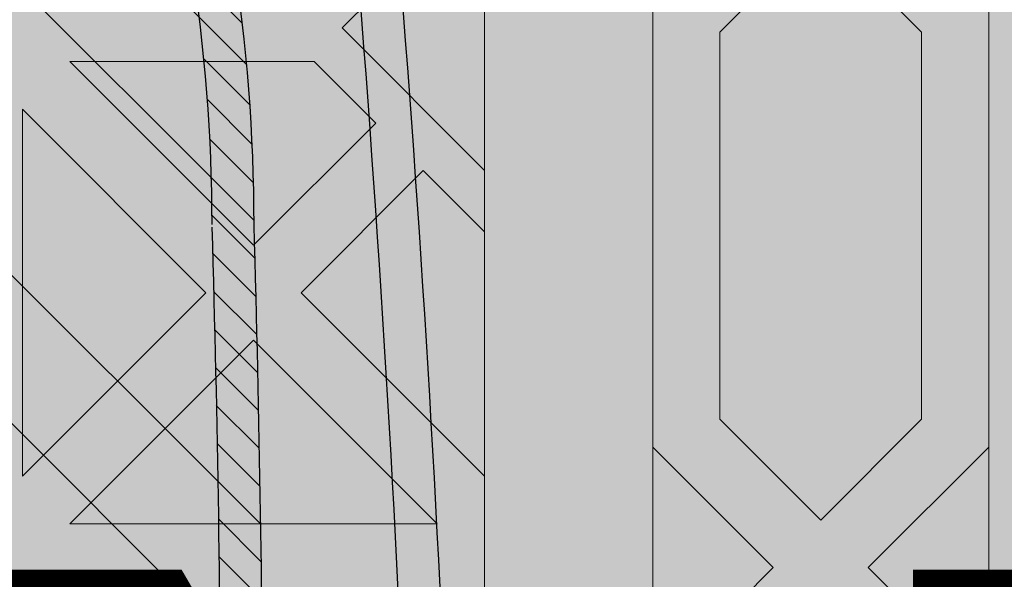
# Model space of a CAD drawing. Units: inches. Extents: x 844 to 2234, y 346 to 1084.
# Tile 84 of 93: x 2006.557 to 2010.294, y 704.373 to 706.497. Entities that reach past the tile are written whole.
import ezdxf

# ---------------------------------------------------------------- set-up
doc = ezdxf.new("R2010")
doc.units = ezdxf.units.IN
doc.header["$MEASUREMENT"] = 0
for name, color, linetype, lineweight in [('A-ANNO-DIMS', 2, 'Continuous', 18), ('furniture', 8, 'Continuous', 18), ('RA-AP-01$0$INT', 35, 'Continuous', 5)]:
    doc.layers.add(name, color=color, linetype=linetype, lineweight=lineweight)
doc.layers.add('RA-AP-01$0$FURN', color=3, linetype='Continuous')
doc.layers.add('RA-AP-01$0$WOOD', color=64, linetype='Continuous')
doc.styles.get("Standard").update_dxf_attribs({"font": 'arial.ttf'})
doc.dimstyles.get("Standard").update_dxf_attribs({"dimtxt": 6, "dimasz": 3, "dimexe": 0.18, "dimexo": 0.0625, "dimgap": 0.09, "dimtad": 0, "dimtih": 1, "dimtoh": 1, "dimdec": 1, "dimzin": 0, "dimdsep": 46, "dimlunit": 3, "dimtxsty": 'Standard', "dimblk": 'ARCHTICK', "dimcen": 0.09, "dimadec": 0, "dimazin": 0, "dimtfac": 1, "dimtdec": 1, "dimtofl": 0, "dimtmove": 0, "dimatfit": 3, "dimfxl": 1, "dimtolj": 1, "dimtzin": 0, "dimarcsym": 0})

# ---------------------------------------------------------------- blocks, each defined once
blk = doc.blocks.new('A$C18D01794')
at = {"layer": 'RA-AP-01$0$INT'}
h = blk.add_hatch(color=256, dxfattribs=at)
h.paths.add_polyline_path([(4.35521, -6.15671), (4.35521, -8.05671), (5.45521, -8.05671), (5.45521, -6.15671)])
h.paths.add_polyline_path([(4.40521, -8.00671), (4.40521, -6.20671), (5.40521, -6.20671), (5.40521, -8.00671)], flags=16)
h = blk.add_hatch(color=256, dxfattribs=at)
h.paths.add_polyline_path([(4.50521, -7.5855), (4.46935, -7.54964), (4.50521, -7.51378), (4.50521, -7.38196), (4.46935, -7.34611), (4.50521, -7.31025), (4.50521, -7.17843), (4.46935, -7.14257), (4.50521, -7.10671), (4.47692, -7.10671), (4.45521, -7.12843), (4.43349, -7.10671), (4.40521, -7.10671), (4.44106, -7.14257), (4.40521, -7.17843), (4.40521, -7.31025), (4.44106, -7.34611), (4.40521, -7.38196), (4.40521, -7.51378), (4.44106, -7.54964), (4.40521, -7.5855), (4.40521, -7.71732), (4.44106, -7.75318), (4.40521, -7.78903), (4.40521, -8.00671), (4.64435, -8.00671), (4.68021, -7.97085), (4.71606, -8.00671), (4.86935, -8.00671), (4.90521, -7.97085), (4.94106, -8.00671), (5.09435, -8.00671), (5.13021, -7.97085), (5.16606, -8.00671), (5.40521, -8.00671), (5.40521, -7.78903), (5.36935, -7.75318), (5.40521, -7.71732), (5.40521, -7.5855), (5.36935, -7.54964), (5.40521, -7.51378), (5.40521, -7.38196), (5.36935, -7.34611), (5.40521, -7.31025), (5.40521, -7.17843), (5.36935, -7.14257), (5.40521, -7.10671), (5.37692, -7.10671), (5.35521, -7.12843), (5.33349, -7.10671), (5.30521, -7.10671), (5.34106, -7.14257), (5.30521, -7.17843), (5.30521, -7.31025), (5.34106, -7.34611), (5.30521, -7.38196), (5.30521, -7.51378), (5.34106, -7.54964), (5.30521, -7.5855), (5.30521, -7.71732), (5.34106, -7.75318), (5.30521, -7.78903), (5.30521, -7.90671), (5.16606, -7.90671), (5.13021, -7.94257), (5.09435, -7.90671), (4.94106, -7.90671), (4.90521, -7.94257), (4.86935, -7.90671), (4.71606, -7.90671), (4.68021, -7.94257), (4.64435, -7.90671), (4.50521, -7.90671), (4.50521, -7.78903), (4.46935, -7.75318), (4.50521, -7.71732)])
h.paths.add_polyline_path([(4.48521, -7.70903), (4.45521, -7.73903), (4.42521, -7.70903), (4.42521, -7.59378), (4.45521, -7.56378), (4.48521, -7.59378)], flags=16)
h.paths.add_polyline_path([(4.45521, -7.76732), (4.48521, -7.79732), (4.48521, -7.91257), (4.45521, -7.94257), (4.42521, -7.91257), (4.42521, -7.79732)], flags=16)
h.paths.add_polyline_path([(4.45521, -7.5355), (4.42521, -7.5055), (4.42521, -7.39025), (4.45521, -7.36025), (4.48521, -7.39025), (4.48521, -7.5055)], flags=16)
h.paths.add_polyline_path([(4.49935, -7.92671), (4.63606, -7.92671), (4.66606, -7.95671), (4.63606, -7.98671), (4.49935, -7.98671), (4.46935, -7.95671)], flags=16)
h.paths.add_polyline_path([(4.42521, -7.94085), (4.47106, -7.98671), (4.42521, -7.98671)], flags=16)
h.paths.add_polyline_path([(4.45521, -7.33196), (4.42521, -7.30196), (4.42521, -7.18671), (4.45521, -7.15671), (4.48521, -7.18671), (4.48521, -7.30196)], flags=16)
h.paths.add_polyline_path([(4.72435, -7.92671), (4.86106, -7.92671), (4.89106, -7.95671), (4.86106, -7.98671), (4.72435, -7.98671), (4.69435, -7.95671)], flags=16)
h.paths.add_polyline_path([(4.91935, -7.95671), (4.94935, -7.92671), (5.08606, -7.92671), (5.11606, -7.95671), (5.08606, -7.98671), (4.94935, -7.98671)], flags=16)
h.paths.add_polyline_path([(5.14435, -7.95671), (5.17435, -7.92671), (5.31106, -7.92671), (5.34106, -7.95671), (5.31106, -7.98671), (5.17435, -7.98671)], flags=16)
h.paths.add_polyline_path([(5.32521, -7.59378), (5.35521, -7.56378), (5.38521, -7.59378), (5.38521, -7.70903), (5.35521, -7.73903), (5.32521, -7.70903)], flags=16)
h.paths.add_polyline_path([(5.32521, -7.79732), (5.35521, -7.76732), (5.38521, -7.79732), (5.38521, -7.91257), (5.35521, -7.94257), (5.32521, -7.91257)], flags=16)
h.paths.add_polyline_path([(5.32521, -7.5055), (5.32521, -7.39025), (5.35521, -7.36025), (5.38521, -7.39025), (5.38521, -7.5055), (5.35521, -7.5355)], flags=16)
h.paths.add_polyline_path([(5.32521, -7.30196), (5.32521, -7.18671), (5.35521, -7.15671), (5.38521, -7.18671), (5.38521, -7.30196), (5.35521, -7.33196)], flags=16)
h.paths.add_polyline_path([(5.33935, -7.98671), (5.38521, -7.94085), (5.38521, -7.98671)], flags=16)
h = blk.add_hatch(color=256, dxfattribs=at)
h.paths.add_polyline_path([(4.46935, -7.14257), (4.50521, -7.17843), (4.50521, -7.10671)])
h.paths.add_polyline_path([(4.45521, -7.12843), (4.47692, -7.10671), (4.43349, -7.10671)])
h.paths.add_polyline_path([(4.40521, -7.17843), (4.44106, -7.14257), (4.40521, -7.10671)])
h.paths.add_polyline_path([(4.42521, -7.30196), (4.45521, -7.33196), (4.48521, -7.30196), (4.48521, -7.18671), (4.45521, -7.15671), (4.42521, -7.18671)])
h.paths.add_polyline_path([(4.50521, -7.38196), (4.50521, -7.31025), (4.46935, -7.34611)])
h.paths.add_polyline_path([(4.42521, -7.5055), (4.45521, -7.5355), (4.48521, -7.5055), (4.48521, -7.39025), (4.45521, -7.36025), (4.42521, -7.39025)])
h.paths.add_polyline_path([(4.42521, -7.70903), (4.45521, -7.73903), (4.48521, -7.70903), (4.48521, -7.59378), (4.45521, -7.56378), (4.42521, -7.59378)])
h.paths.add_polyline_path([(4.46935, -7.54964), (4.50521, -7.5855), (4.50521, -7.51378)])
h.paths.add_polyline_path([(4.40521, -7.5855), (4.44106, -7.54964), (4.40521, -7.51378)])
h.paths.add_polyline_path([(4.40521, -7.78903), (4.44106, -7.75318), (4.40521, -7.71732)])
h.paths.add_polyline_path([(4.46935, -7.75318), (4.50521, -7.78903), (4.50521, -7.71732)])
h.paths.add_polyline_path([(4.42521, -7.91257), (4.45521, -7.94257), (4.48521, -7.91257), (4.48521, -7.79732), (4.45521, -7.76732), (4.42521, -7.79732)])
h.paths.add_polyline_path([(4.42521, -7.98671), (4.47106, -7.98671), (4.42521, -7.94085)])
h.paths.add_polyline_path([(4.49935, -7.98671), (4.63606, -7.98671), (4.66606, -7.95671), (4.63606, -7.92671), (4.49935, -7.92671), (4.46935, -7.95671)])
h.paths.add_polyline_path([(4.68021, -7.94257), (4.71606, -7.90671), (4.64435, -7.90671)])
h.paths.add_polyline_path([(4.64435, -8.00671), (4.71606, -8.00671), (4.68021, -7.97085)])
h.paths.add_polyline_path([(4.72435, -7.98671), (4.86106, -7.98671), (4.89106, -7.95671), (4.86106, -7.92671), (4.72435, -7.92671), (4.69435, -7.95671)])
h.paths.add_polyline_path([(4.90521, -7.94257), (4.94106, -7.90671), (4.86935, -7.90671)])
h.paths.add_polyline_path([(4.86935, -8.00671), (4.94106, -8.00671), (4.90521, -7.97085)])
h.paths.add_polyline_path([(4.94935, -7.98671), (5.08606, -7.98671), (5.11606, -7.95671), (5.08606, -7.92671), (4.94935, -7.92671), (4.91935, -7.95671)])
h.paths.add_polyline_path([(5.13021, -7.94257), (5.16606, -7.90671), (5.09435, -7.90671)])
h.paths.add_polyline_path([(5.09435, -8.00671), (5.16606, -8.00671), (5.13021, -7.97085)])
h.paths.add_polyline_path([(5.17435, -7.98671), (5.31106, -7.98671), (5.34106, -7.95671), (5.31106, -7.92671), (5.17435, -7.92671), (5.14435, -7.95671)])
h.paths.add_polyline_path([(5.32521, -7.91257), (5.35521, -7.94257), (5.38521, -7.91257), (5.38521, -7.79732), (5.35521, -7.76732), (5.32521, -7.79732)])
h.paths.add_polyline_path([(5.33935, -7.98671), (5.38521, -7.98671), (5.38521, -7.94085)])
h.paths.add_polyline_path([(5.32521, -7.70903), (5.35521, -7.73903), (5.38521, -7.70903), (5.38521, -7.59378), (5.35521, -7.56378), (5.32521, -7.59378)])
h.paths.add_polyline_path([(5.30521, -7.78903), (5.34106, -7.75318), (5.30521, -7.71732)])
h.paths.add_polyline_path([(5.36935, -7.75318), (5.40521, -7.78903), (5.40521, -7.71732)])
h.paths.add_polyline_path([(5.40521, -7.5855), (5.40521, -7.51378), (5.36935, -7.54964)])
h.paths.add_polyline_path([(5.30521, -7.5855), (5.34106, -7.54964), (5.30521, -7.51378)])
h.paths.add_polyline_path([(5.32521, -7.5055), (5.35521, -7.5355), (5.38521, -7.5055), (5.38521, -7.39025), (5.35521, -7.36025), (5.32521, -7.39025)])
h.paths.add_polyline_path([(5.30521, -7.38196), (5.34106, -7.34611), (5.30521, -7.31025)])
h.paths.add_polyline_path([(5.32521, -7.30196), (5.35521, -7.33196), (5.38521, -7.30196), (5.38521, -7.18671), (5.35521, -7.15671), (5.32521, -7.18671)])
h.paths.add_polyline_path([(5.40458, -7.38134, -0.001218), (5.40521, -7.38111), (5.40521, -7.31025), (5.36935, -7.34611)])
h.paths.add_polyline_path([(5.36935, -7.14257), (5.40521, -7.17843), (5.40521, -7.10671)])
h.paths.add_polyline_path([(5.35521, -7.12843), (5.37692, -7.10671), (5.33349, -7.10671)])
h.paths.add_polyline_path([(5.30521, -7.17843), (5.34106, -7.14257), (5.30521, -7.10671)])
for points in [[(4.50521, -7.90671), (5.30521, -7.90671), (5.30521, -7.10671), (5.25521, -7.10671), (5.25521, -7.85671), (4.55521, -7.85671), (4.55521, -7.10671), (4.50521, -7.10671)], [(4.40521, -7.38196), (4.44106, -7.34611), (4.40521, -7.31025)]]:
    blk.add_hatch(color=256, dxfattribs=at).paths.add_polyline_path(points)
h = blk.add_hatch(color=256, dxfattribs=at)
h.paths.add_polyline_path([(4.58592, -7.85671), (4.6142, -7.85671), (4.66885, -7.80207), (4.72349, -7.85671), (4.77177, -7.85671), (4.82642, -7.80207), (4.86278, -7.83843), (4.8445, -7.85671), (4.86278, -7.85671), (4.90521, -7.81429), (4.94763, -7.85671), (4.96592, -7.85671), (4.94763, -7.83843), (4.98399, -7.80207), (5.03864, -7.85671), (5.08692, -7.85671), (5.14157, -7.80207), (5.19621, -7.85671), (5.2245, -7.85671), (4.90521, -7.53742)])
h.paths.add_polyline_path([(4.89521, -7.57571), (4.89521, -7.685), (4.84056, -7.63035)], flags=16)
h.paths.add_polyline_path([(4.91521, -7.57571), (4.96985, -7.63035), (4.91521, -7.685)], flags=16)
h.paths.add_polyline_path([(4.82642, -7.64449), (4.88106, -7.69914), (4.77177, -7.69914)], flags=16)
h.paths.add_polyline_path([(4.98399, -7.64449), (5.03864, -7.69914), (4.92935, -7.69914)], flags=16)
h.paths.add_polyline_path([(4.88106, -7.71914), (4.82642, -7.77378), (4.77177, -7.71914)], flags=16)
h.paths.add_polyline_path([(4.92935, -7.71914), (5.03864, -7.71914), (4.98399, -7.77378)], flags=16)
h.paths.add_polyline_path([(4.89521, -7.73328), (4.89521, -7.806), (4.87692, -7.82429), (4.84056, -7.78793)], flags=16)
h.paths.add_polyline_path([(4.91521, -7.73328), (4.96985, -7.78793), (4.93349, -7.82429), (4.91521, -7.806)], flags=16)
h.paths.add_polyline_path([(4.75763, -7.73328), (4.81228, -7.78793), (4.75763, -7.84257)], flags=16)
h.paths.add_polyline_path([(4.73763, -7.73328), (4.73763, -7.84257), (4.68299, -7.78793)], flags=16)
h.paths.add_polyline_path([(5.05278, -7.73328), (5.05278, -7.84257), (4.99814, -7.78793)], flags=16)
h.paths.add_polyline_path([(5.07278, -7.73328), (5.12742, -7.78793), (5.07278, -7.84257)], flags=16)
h.paths.add_polyline_path([(4.93592, -7.50671), (5.25521, -7.826), (5.25521, -7.79772), (5.20056, -7.74307), (5.25521, -7.68843), (5.25521, -7.64014), (5.20056, -7.5855), (5.23692, -7.54914), (5.25521, -7.56742), (5.25521, -7.54914), (5.21278, -7.50671), (5.25521, -7.46429), (5.25521, -7.446), (5.23692, -7.46429), (5.20056, -7.42793), (5.25521, -7.37328), (5.25521, -7.325), (5.20056, -7.27035), (5.25521, -7.21571), (5.25521, -7.18742)])
h.paths.add_polyline_path([(5.04299, -7.42793), (5.09763, -7.37328), (5.09763, -7.48257)], flags=16)
h.paths.add_polyline_path([(5.02885, -7.44207), (5.08349, -7.49671), (4.9742, -7.49671)], flags=16)
h.paths.add_polyline_path([(5.11763, -7.37328), (5.17228, -7.42793), (5.11763, -7.48257)], flags=16)
h.paths.add_polyline_path([(5.08349, -7.51671), (5.02885, -7.57136), (4.9742, -7.51671)], flags=16)
h.paths.add_polyline_path([(5.13177, -7.35914), (5.18642, -7.41378), (5.24106, -7.35914)], flags=17)
h.paths.add_polyline_path([(5.13177, -7.49671), (5.18642, -7.44207), (5.22278, -7.47843), (5.2045, -7.49671)], flags=16)
h.paths.add_polyline_path([(5.09763, -7.53085), (5.09763, -7.64014), (5.04299, -7.5855)], flags=16)
h.paths.add_polyline_path([(5.13177, -7.33914), (5.24106, -7.33914), (5.18642, -7.28449)], flags=17)
h.paths.add_polyline_path([(5.13177, -7.51671), (5.2045, -7.51671), (5.22278, -7.535), (5.18642, -7.57136)], flags=16)
h.paths.add_polyline_path([(5.11763, -7.53085), (5.17228, -7.5855), (5.11763, -7.64014)], flags=16)
h.paths.add_polyline_path([(5.18642, -7.59964), (5.24106, -7.65429), (5.13177, -7.65429)], flags=16)
h.paths.add_polyline_path([(5.13177, -7.67429), (5.24106, -7.67429), (5.18642, -7.72893)], flags=16)
h.paths.add_polyline_path([(5.25521, -7.126), (5.25521, -7.10671), (4.55521, -7.10671), (4.55521, -7.126), (4.90521, -7.476)])
h.paths.add_polyline_path([(4.98399, -7.36893), (4.92935, -7.31429), (5.03864, -7.31429)], flags=16)
h.paths.add_polyline_path([(4.96985, -7.38307), (4.91521, -7.43772), (4.91521, -7.32843)], flags=16)
h.paths.add_polyline_path([(4.92935, -7.29429), (4.98399, -7.23964), (5.03864, -7.29429)], flags=16)
h.paths.add_polyline_path([(5.05278, -7.28014), (4.99814, -7.2255), (5.05278, -7.17085)], flags=16)
h.paths.add_polyline_path([(5.07278, -7.28014), (5.07278, -7.17085), (5.12742, -7.2255)], flags=16)
h.paths.add_polyline_path([(4.89521, -7.43772), (4.84056, -7.38307), (4.89521, -7.32843)], flags=16)
h.paths.add_polyline_path([(4.91521, -7.28014), (4.91521, -7.20742), (4.93349, -7.18914), (4.96985, -7.2255)], flags=16)
h.paths.add_polyline_path([(4.88106, -7.31429), (4.82642, -7.36893), (4.77177, -7.31429)], flags=16)
h.paths.add_polyline_path([(4.89521, -7.28014), (4.84056, -7.2255), (4.87692, -7.18914), (4.89521, -7.20742)], flags=16)
h.paths.add_polyline_path([(4.98399, -7.21136), (4.94763, -7.175), (4.96592, -7.15671), (5.03864, -7.15671)], flags=16)
h.paths.add_polyline_path([(4.88106, -7.29429), (4.77177, -7.29429), (4.82642, -7.23964)], flags=16)
h.paths.add_polyline_path([(4.90521, -7.19914), (4.86278, -7.15671), (4.94763, -7.15671)], flags=16)
h.paths.add_polyline_path([(5.14157, -7.21136), (5.08692, -7.15671), (5.19621, -7.15671)], flags=16)
h.paths.add_polyline_path([(4.82642, -7.21136), (4.77177, -7.15671), (4.8445, -7.15671), (4.86278, -7.175)], flags=16)
h.paths.add_polyline_path([(4.81228, -7.2255), (4.75763, -7.28014), (4.75763, -7.17085)], flags=16)
h.paths.add_polyline_path([(4.73763, -7.28014), (4.68299, -7.2255), (4.73763, -7.17085)], flags=16)
h.paths.add_polyline_path([(4.72349, -7.15671), (4.66885, -7.21136), (4.6142, -7.15671)], flags=16)
h.paths.add_polyline_path([(4.59763, -7.50671), (4.55521, -7.54914), (4.55521, -7.56742), (4.57349, -7.54914), (4.60985, -7.5855), (4.55521, -7.64014), (4.55521, -7.68843), (4.60985, -7.74307), (4.55521, -7.79772), (4.55521, -7.826), (4.8745, -7.50671), (4.55521, -7.18742), (4.55521, -7.21571), (4.60985, -7.27035), (4.55521, -7.325), (4.55521, -7.37328), (4.60985, -7.42793), (4.57349, -7.46429), (4.55521, -7.446), (4.55521, -7.46429)])
h.paths.add_polyline_path([(4.71278, -7.48257), (4.71278, -7.37328), (4.76742, -7.42793)], flags=16)
h.paths.add_polyline_path([(4.72692, -7.49671), (4.78157, -7.44207), (4.83621, -7.49671)], flags=16)
h.paths.add_polyline_path([(4.69278, -7.48257), (4.63814, -7.42793), (4.69278, -7.37328)], flags=16)
h.paths.add_polyline_path([(4.72692, -7.51671), (4.83621, -7.51671), (4.78157, -7.57136)], flags=16)
h.paths.add_polyline_path([(4.67864, -7.49671), (4.60592, -7.49671), (4.58763, -7.47843), (4.62399, -7.44207)], flags=16)
h.paths.add_polyline_path([(4.71278, -7.53085), (4.76742, -7.5855), (4.71278, -7.64014)], flags=16)
h.paths.add_polyline_path([(4.67864, -7.51671), (4.62399, -7.57136), (4.58763, -7.535), (4.60592, -7.51671)], flags=16)
h.paths.add_polyline_path([(4.69278, -7.53085), (4.69278, -7.64014), (4.63814, -7.5855)], flags=16)
h.paths.add_polyline_path([(4.62399, -7.41378), (4.67864, -7.35914), (4.56935, -7.35914)], flags=17)
h.paths.add_polyline_path([(4.62399, -7.59964), (4.67864, -7.65429), (4.56935, -7.65429)], flags=16)
h.paths.add_polyline_path([(4.67864, -7.33914), (4.62399, -7.28449), (4.56935, -7.33914)], flags=17)
h.paths.add_polyline_path([(4.67864, -7.67429), (4.62399, -7.72893), (4.56935, -7.67429)], flags=16)
h = blk.add_hatch(color=256, dxfattribs=at)
h.paths.add_polyline_path([(4.78157, -7.44207), (4.83621, -7.49671), (4.72692, -7.49671)])
h.paths.add_polyline_path([(4.83621, -7.51671), (4.78157, -7.57136), (4.72692, -7.51671)])
h.paths.add_polyline_path([(4.76742, -7.5855), (4.71278, -7.64014), (4.71278, -7.53085)])
h.paths.add_polyline_path([(4.69278, -7.53085), (4.69278, -7.64014), (4.63814, -7.5855)])
h.paths.add_polyline_path([(4.67864, -7.51671), (4.62399, -7.57136), (4.58763, -7.535), (4.60592, -7.51671)])
h.paths.add_polyline_path([(4.57349, -7.54914), (4.60985, -7.5855), (4.55521, -7.64014), (4.55521, -7.56742)])
h.paths.add_polyline_path([(4.62399, -7.59964), (4.67864, -7.65429), (4.56935, -7.65429)])
h.paths.add_polyline_path([(4.67864, -7.67429), (4.62399, -7.72893), (4.56935, -7.67429)])
h.paths.add_polyline_path([(4.60985, -7.74307), (4.55521, -7.79772), (4.55521, -7.68843)])
h.paths.add_polyline_path([(4.59763, -7.50671), (4.55521, -7.54914), (4.55521, -7.46429)])
h.paths.add_polyline_path([(4.67864, -7.49671), (4.60592, -7.49671), (4.58763, -7.47843), (4.62399, -7.44207)])
h.paths.add_polyline_path([(4.69278, -7.37328), (4.69278, -7.48257), (4.63814, -7.42793)])
h.paths.add_polyline_path([(4.76742, -7.42793), (4.71278, -7.48257), (4.71278, -7.37328)])
h.paths.add_polyline_path([(4.67864, -7.35914), (4.62399, -7.41378), (4.56935, -7.35914)])
h.paths.add_polyline_path([(4.60985, -7.42793), (4.57349, -7.46429), (4.55521, -7.446), (4.55521, -7.37328)])
h.paths.add_polyline_path([(4.62399, -7.28449), (4.67864, -7.33914), (4.56935, -7.33914)])
h.paths.add_polyline_path([(4.60985, -7.27035), (4.55521, -7.325), (4.55521, -7.21571)])
for p, q in [((4.55521, -7.10671), (4.55521, -7.85671)), ((4.40521, -7.31025), (4.44106, -7.34611)), ((4.50521, -7.31025), (4.46935, -7.34611)), ((4.40521, -7.38196), (4.44106, -7.34611)), ((4.50521, -7.38196), (4.46935, -7.34611)), ((4.67864, -7.35914), (4.56935, -7.35914)), ((4.56935, -7.35914), (4.62399, -7.41378)), ((4.67864, -7.35914), (4.62399, -7.41378)), ((4.42521, -7.39025), (4.45521, -7.36025)), ((4.48521, -7.39025), (4.45521, -7.36025)), ((4.55521, -7.446), (4.55521, -7.37328)), ((4.55521, -7.37328), (4.60985, -7.42793)), ((4.69278, -7.37328), (4.63814, -7.42793)), ((4.69278, -7.37328), (4.69278, -7.48257)), ((4.42521, -7.39025), (4.42521, -7.5055)), ((4.48521, -7.39025), (4.48521, -7.5055)), ((4.60985, -7.42793), (4.57349, -7.46429)), ((4.69278, -7.48257), (4.63814, -7.42793)), ((4.62399, -7.44207), (4.58763, -7.47843)), ((4.67864, -7.49671), (4.62399, -7.44207)), ((4.55521, -7.446), (4.57349, -7.46429)), ((4.57349, -7.46429), (4.55521, -7.446)), ((4.59763, -7.50671), (4.55521, -7.46429)), ((4.55521, -7.46429), (4.55521, -7.54914)), ((4.60592, -7.49671), (4.58763, -7.47843)), ((4.60592, -7.49671), (4.67864, -7.49671)), ((4.42521, -7.5055), (4.45521, -7.5355)), ((4.48521, -7.5055), (4.45521, -7.5355)), ((4.59763, -7.50671), (4.55521, -7.54914))]:
    blk.add_line(p, q, dxfattribs=at)
for points in [[(5.40521, -8.00671), (4.40521, -8.00671), (4.40521, -7.10671)], [(5.30521, -7.10671), (5.30521, -7.90671), (4.50521, -7.90671), (4.50521, -7.10671)]]:
    blk.add_lwpolyline(points, dxfattribs=at)
blk = doc.blocks.new('A$C32926AE1')
at = {"layer": 'RA-AP-01$0$WOOD'}
h = blk.add_hatch(color=256, dxfattribs=at)
h.dxf.hatch_style = 1
h.paths.add_polyline_path([(5.15743, 4.57348, -0.100949), (5.1554, 4.59337, -0.184266), (5.17225, 4.6388, 0.205661), (5.17956, 4.66132, 0.361434), (5.13435, 4.70652, 0.205661), (5.11183, 4.69921, -0.184266), (5.0664, 4.68237, -0.105531), (5.04566, 4.68467, 0.156764), (4.76389, 4.68467, -0.105531), (4.74314, 4.68237, -0.184266), (4.69771, 4.69921, 0.205661), (4.67519, 4.70652, 0.361434), (4.62998, 4.66132, 0.205661), (4.63729, 4.6388, -0.184266), (4.65414, 4.59337, -0.100949), (4.65211, 4.57348, 0.02141), (4.62975, 4.15671, 0.02141), (4.65211, 3.73994, -0.100949), (4.65414, 3.72006, -0.184266), (4.63729, 3.67463, 0.205661), (4.62998, 3.65211, 0.361434), (4.67519, 3.6069, 0.205661), (4.69771, 3.61421, -0.184266), (4.74314, 3.63106, -0.105531), (4.76389, 3.62875, 0.156764), (5.04566, 3.62875, -0.105531), (5.0664, 3.63106, -0.184266), (5.11183, 3.61421, 0.205661), (5.13435, 3.6069, 0.361434), (5.17956, 3.65211, 0.205661), (5.17225, 3.67463, -0.184266), (5.1554, 3.72006, -0.100949), (5.15743, 3.73994, 0.02141), (5.17979, 4.15671, 0.02141)])
h.paths.add_polyline_path([(4.63975, 4.15671, 0.021354), (4.66197, 3.74189, -0.094076), (4.66414, 3.71961, -0.182482), (4.64481, 3.66804, 0.205661), (4.63994, 3.65302, 0.361434), (4.67611, 3.61686, 0.205661), (4.69112, 3.62173, -0.182482), (4.7427, 3.64106, -0.102989), (4.76699, 3.63826, 0.156709), (5.04255, 3.63826, -0.102989), (5.06685, 3.64106, -0.182482), (5.11842, 3.62173, 0.205661), (5.13344, 3.61686, 0.361434), (5.1696, 3.65302, 0.205661), (5.16473, 3.66804, -0.182482), (5.1454, 3.71961, -0.094076), (5.14757, 3.74189, 0.021354), (5.16979, 4.15671, 0.021354), (5.14757, 4.57154, -0.094076), (5.1454, 4.59381, -0.182482), (5.16473, 4.64539, 0.205661), (5.1696, 4.6604, 0.361434), (5.13344, 4.69657, 0.205661), (5.11842, 4.69169, -0.182482), (5.06685, 4.67236, -0.102989), (5.04255, 4.67517, 0.156709), (4.76699, 4.67517, -0.102989), (4.7427, 4.67236, -0.182482), (4.69112, 4.69169, 0.205661), (4.67611, 4.69657, 0.361434), (4.63994, 4.6604, 0.205661), (4.64481, 4.64539, -0.182482), (4.66414, 4.59381, -0.094076), (4.66197, 4.57154, 0.021354)], flags=16)
h.paths.add_polyline_path([(5.12979, 4.43217, -0.014166), (5.13015, 4.15693, -0.014166), (5.12979, 3.88169, -0.078525), (5.1098, 3.75514, 0.094597), (5.10541, 3.7179, 0.104317), (5.11607, 3.67039, 0.104317), (5.06856, 3.68105, 0.094597), (5.03132, 3.67666, -0.158024), (4.77823, 3.67666, 0.094597), (4.74098, 3.68105, 0.104317), (4.69347, 3.67039, 0.104317), (4.70413, 3.7179, 0.094597), (4.69975, 3.75514, -0.078525), (4.67975, 3.88169, -0.014166), (4.67939, 4.15693, -0.014166), (4.67975, 4.43217, -0.078525), (4.69975, 4.55871, 0.094597), (4.70413, 4.59596, 0.104317), (4.69347, 4.64347, 0.104317), (4.74098, 4.6328, 0.094597), (4.77823, 4.63719, -0.158024), (5.03132, 4.63719, 0.094597), (5.06856, 4.6328, 0.104317), (5.11607, 4.64347, 0.104317), (5.10541, 4.59596, 0.094597), (5.1098, 4.55871, -0.078525)], flags=0)
h.paths.add_polyline_path([(5.11979, 4.43226, -0.0142), (5.12016, 4.15693, -0.0142), (5.11979, 3.8816, -0.078489), (5.10027, 3.75819, 0.094014), (5.09541, 3.71748, 0.060627), (5.09962, 3.68684, 0.060627), (5.06898, 3.69105, 0.094014), (5.02827, 3.68619, -0.158071), (4.78127, 3.68619, 0.094014), (4.74056, 3.69105, 0.060627), (4.70993, 3.68684, 0.060627), (4.71413, 3.71748, 0.094014), (4.70927, 3.75819, -0.078489), (4.68975, 3.8816, -0.0142), (4.68939, 4.15693, -0.0142), (4.68975, 4.43226, -0.078489), (4.70927, 4.55566, 0.094014), (4.71413, 4.59638, 0.060627), (4.70993, 4.62701, 0.060627), (4.74056, 4.62281, 0.094014), (4.78127, 4.62767, -0.158071), (5.02827, 4.62767, 0.094014), (5.06898, 4.62281, 0.060627), (5.09962, 4.62701, 0.060627), (5.09541, 4.59638, 0.094014), (5.10027, 4.55566, -0.078489)], flags=0)
h.paths.add_polyline_path([(5.06979, 4.43022, -0.014242), (5.07017, 4.15693, -0.014242), (5.06979, 3.88364, -0.080061), (5.05266, 3.77346, 0.052642), (5.04591, 3.74055, 0.052642), (5.013, 3.7338, -0.158303), (4.79655, 3.7338, 0.052642), (4.76363, 3.74055, 0.052642), (4.75688, 3.77346, -0.080061), (4.73975, 3.88364, -0.014242), (4.73937, 4.15693, -0.014242), (4.73975, 4.43022, -0.080061), (4.75688, 4.54039, 0.052642), (4.76363, 4.5733, 0.052642), (4.79655, 4.58006, -0.158303), (5.013, 4.58006, 0.052642), (5.04591, 4.5733, 0.052642), (5.05266, 4.54039, -0.080061)], flags=0)
h.paths.add_polyline_path([(5.04979, 4.43038, -0.01431), (5.05018, 4.15693, -0.01431), (5.04979, 3.88347, -0.080069), (5.03362, 3.77958, 0.030626), (5.02824, 3.75822, 0.030626), (5.00688, 3.75284, -0.158398), (4.80266, 3.75284, 0.030626), (4.7813, 3.75822, 0.030626), (4.77592, 3.77958, -0.080069), (4.75975, 3.88347, -0.01431), (4.75936, 4.15693, -0.01431), (4.75975, 4.43038, -0.080069), (4.77592, 4.53427, 0.030626), (4.7813, 4.55564, 0.030626), (4.80266, 4.56102, -0.158398), (5.00688, 4.56102, 0.030626), (5.02824, 4.55564, 0.030626), (5.03362, 4.53427, -0.080069)], flags=0)
h.paths.add_polyline_path([(4.99977, 4.42817, -0.014344), (5.0002, 4.15693, -0.014344), (4.99977, 3.88568, -0.078464), (4.98736, 3.7991, -0.150605), (4.82219, 3.7991, -0.078464), (4.80978, 3.88568, -0.014344), (4.80934, 4.15693, -0.014344), (4.80978, 4.42817, -0.078464), (4.82219, 4.51475, -0.150605), (4.98736, 4.51475, -0.078464)], flags=0)
h.paths.add_polyline_path([(4.97976, 4.42764, -0.014377), (4.98021, 4.15693, -0.014377), (4.97976, 3.88621, -0.068924), (4.97118, 3.81528, -0.129665), (4.83836, 3.81528, -0.068924), (4.82979, 3.88621, -0.014377), (4.82934, 4.15693, -0.014377), (4.82979, 4.42764, -0.068924), (4.83836, 4.49858, -0.129665), (4.97118, 4.49858, -0.068924)], flags=0)
h = blk.add_hatch(color=256, dxfattribs=at)
h.dxf.hatch_style = 1
h.paths.add_polyline_path([(5.1454, 4.59381, -0.182482), (5.16473, 4.64539, 0.205661), (5.1696, 4.6604, 0.361434), (5.13344, 4.69657, 0.205661), (5.11842, 4.69169, -0.182482), (5.06685, 4.67236, -0.102989), (5.04255, 4.67517, 0.156709), (4.76699, 4.67517, -0.102989), (4.7427, 4.67236, -0.182482), (4.69112, 4.69169, 0.205661), (4.67611, 4.69657, 0.361434), (4.63994, 4.6604, 0.205661), (4.64481, 4.64539, -0.182482), (4.66414, 4.59381, -0.094076), (4.66197, 4.57154, 0.021354), (4.63975, 4.15671, 0.021354), (4.66197, 3.74189, -0.094076), (4.66414, 3.71961, -0.182482), (4.64481, 3.66804, 0.205661), (4.63994, 3.65302, 0.361434), (4.67611, 3.61686, 0.205661), (4.69112, 3.62173, -0.182482), (4.7427, 3.64106, -0.102989), (4.76699, 3.63826, 0.156709), (5.04255, 3.63826, -0.102989), (5.06685, 3.64106, -0.182482), (5.11842, 3.62173, 0.205661), (5.13344, 3.61686, 0.361434), (5.1696, 3.65302, 0.205661), (5.16473, 3.66804, -0.182482), (5.1454, 3.71961, -0.094076), (5.14757, 3.74189, 0.021354), (5.16979, 4.15671, 0.021354), (5.14757, 4.57154, -0.094076)])
h.paths.add_polyline_path([(5.1098, 4.55871, -0.078525), (5.12979, 4.43217, -0.014166), (5.13015, 4.15693, -0.014166), (5.12979, 3.88169, -0.078525), (5.1098, 3.75514, 0.094597), (5.10541, 3.7179, 0.104317), (5.11607, 3.67039, 0.104317), (5.06856, 3.68105, 0.094597), (5.03132, 3.67666, -0.158024), (4.77823, 3.67666, 0.094597), (4.74098, 3.68105, 0.104317), (4.69347, 3.67039, 0.104317), (4.70413, 3.7179, 0.094597), (4.69975, 3.75514, -0.078525), (4.67975, 3.88169, -0.014166), (4.67939, 4.15693, -0.014166), (4.67975, 4.43217, -0.078525), (4.69975, 4.55871, 0.094597), (4.70413, 4.59596, 0.104317), (4.69347, 4.64347, 0.104317), (4.74098, 4.6328, 0.094597), (4.77823, 4.63719, -0.158024), (5.03132, 4.63719, 0.094597), (5.06856, 4.6328, 0.104317), (5.11607, 4.64347, 0.104317), (5.10541, 4.59596, 0.094597)], flags=16)
h.paths.add_polyline_path([(5.10027, 4.55566, -0.078489), (5.11979, 4.43226, -0.0142), (5.12016, 4.15693, -0.0142), (5.11979, 3.8816, -0.078489), (5.10027, 3.75819, 0.094014), (5.09541, 3.71748, 0.060627), (5.09962, 3.68684, 0.060627), (5.06898, 3.69105, 0.094014), (5.02827, 3.68619, -0.158071), (4.78127, 3.68619, 0.094014), (4.74056, 3.69105, 0.060627), (4.70993, 3.68684, 0.060627), (4.71413, 3.71748, 0.094014), (4.70927, 3.75819, -0.078489), (4.68975, 3.8816, -0.0142), (4.68939, 4.15693, -0.0142), (4.68975, 4.43226, -0.078489), (4.70927, 4.55566, 0.094014), (4.71413, 4.59638, 0.060627), (4.70993, 4.62701, 0.060627), (4.74056, 4.62281, 0.094014), (4.78127, 4.62767, -0.158071), (5.02827, 4.62767, 0.094014), (5.06898, 4.62281, 0.060627), (5.09962, 4.62701, 0.060627), (5.09541, 4.59638, 0.094014)], flags=0)
h.paths.add_polyline_path([(5.04591, 4.5733, 0.052642), (5.05266, 4.54039, -0.080061), (5.06979, 4.43022, -0.014242), (5.07017, 4.15693, -0.014242), (5.06979, 3.88364, -0.080061), (5.05266, 3.77346, 0.052642), (5.04591, 3.74055, 0.052642), (5.013, 3.7338, -0.158303), (4.79655, 3.7338, 0.052642), (4.76363, 3.74055, 0.052642), (4.75688, 3.77346, -0.080061), (4.73975, 3.88364, -0.014242), (4.73937, 4.15693, -0.014242), (4.73975, 4.43022, -0.080061), (4.75688, 4.54039, 0.052642), (4.76363, 4.5733, 0.052642), (4.79655, 4.58006, -0.158303), (5.013, 4.58006, 0.052642)], flags=0)
h.paths.add_polyline_path([(5.02824, 4.55564, 0.030626), (5.03362, 4.53427, -0.080069), (5.04979, 4.43038, -0.01431), (5.05018, 4.15693, -0.01431), (5.04979, 3.88347, -0.080069), (5.03362, 3.77958, 0.030626), (5.02824, 3.75822, 0.030626), (5.00688, 3.75284, -0.158398), (4.80266, 3.75284, 0.030626), (4.7813, 3.75822, 0.030626), (4.77592, 3.77958, -0.080069), (4.75975, 3.88347, -0.01431), (4.75936, 4.15693, -0.01431), (4.75975, 4.43038, -0.080069), (4.77592, 4.53427, 0.030626), (4.7813, 4.55564, 0.030626), (4.80266, 4.56102, -0.158398), (5.00688, 4.56102, 0.030626)], flags=0)
h.paths.add_polyline_path([(4.98736, 4.51475, -0.078464), (4.99977, 4.42817, -0.014344), (5.0002, 4.15693, -0.014344), (4.99977, 3.88568, -0.078464), (4.98736, 3.7991, -0.150605), (4.82219, 3.7991, -0.078464), (4.80978, 3.88568, -0.014344), (4.80934, 4.15693, -0.014344), (4.80978, 4.42817, -0.078464), (4.82219, 4.51475, -0.150605)], flags=0)
h.paths.add_polyline_path([(4.97118, 4.49858, -0.068924), (4.97976, 4.42764, -0.014377), (4.98021, 4.15693, -0.014377), (4.97976, 3.88621, -0.068924), (4.97118, 3.81528, -0.129665), (4.83836, 3.81528, -0.068924), (4.82979, 3.88621, -0.014377), (4.82934, 4.15693, -0.014377), (4.82979, 4.42764, -0.068924), (4.83836, 4.49858, -0.129665)], flags=0)
h = blk.add_hatch(dxfattribs=at)
h.set_pattern_fill('ANSI31', color=256, scale=0.05, style=0)
h.paths.add_polyline_path([(5.13015, 4.15693, 0.014166), (5.12979, 4.43217, 0.077783), (5.11017, 4.55756, -0.097652), (5.10541, 4.59596, -0.104317), (5.11607, 4.64347), (5.09962, 4.62701, 0.060627), (5.09541, 4.59638, 0.094014), (5.10027, 4.55566, -0.078489), (5.11979, 4.43226, -0.0142), (5.12016, 4.15693, -0.0142), (5.11979, 3.8816, -0.078489), (5.10027, 3.75819, 0.094014), (5.09541, 3.71748, 0.060627), (5.09962, 3.68684), (5.11607, 3.67039, -0.104317), (5.10541, 3.7179, -0.097652), (5.11017, 3.7563, 0.077783), (5.12979, 3.88169, 0.014166)])
h.paths.add_polyline_path([(5.03016, 3.67629, -0.097652), (5.06856, 3.68105, -0.104317), (5.11607, 3.67039), (5.09962, 3.68684, 0.060627), (5.06898, 3.69105, 0.094014), (5.02827, 3.68619, -0.158071), (4.78127, 3.68619, 0.094014), (4.74056, 3.69105, 0.060627), (4.70993, 3.68684), (4.69347, 3.67039, -0.104317), (4.74098, 3.68105, -0.097652), (4.77938, 3.67629, 0.156513)])
h.paths.add_polyline_path([(4.68975, 3.8816, -0.0142), (4.68939, 4.15693, -0.0142), (4.68975, 4.43226, -0.078489), (4.70927, 4.55566, 0.094014), (4.71413, 4.59638, 0.060627), (4.70993, 4.62701), (4.69347, 4.64347, -0.104317), (4.70413, 4.59596, -0.097652), (4.69937, 4.55756, 0.077783), (4.67975, 4.43217, 0.014166), (4.67939, 4.15693, 0.014166), (4.67975, 3.88169, 0.077783), (4.69937, 3.7563, -0.097652), (4.70413, 3.7179, -0.104317), (4.69347, 3.67039), (4.70993, 3.68684, 0.060627), (4.71413, 3.71748, 0.094014), (4.70927, 3.75819, -0.078489)])
h.paths.add_polyline_path([(4.77938, 4.63756, -0.097652), (4.74098, 4.6328, -0.104317), (4.69347, 4.64347), (4.70993, 4.62701, 0.060627), (4.74056, 4.62281, 0.094014), (4.78127, 4.62767, -0.158071), (5.02827, 4.62767, 0.094014), (5.06898, 4.62281, 0.060627), (5.09962, 4.62701), (5.11607, 4.64347, -0.104317), (5.06856, 4.6328, -0.097652), (5.03016, 4.63756, 0.156513)])
h = blk.add_hatch(dxfattribs=at)
h.set_pattern_fill('ANSI32', color=256, scale=0.2, style=0)
h.paths.add_polyline_path([(5.11979, 4.43226, 0.077702), (5.10066, 4.55447, -0.09689), (5.09541, 4.59638, -0.060627), (5.09962, 4.62701, -0.060627), (5.06898, 4.62281, -0.09689), (5.02707, 4.62805, 0.156466), (4.78247, 4.62805, -0.09689), (4.74056, 4.62281, -0.060627), (4.70993, 4.62701, -0.060627), (4.71413, 4.59638, -0.09689), (4.70888, 4.55447, 0.077702), (4.68975, 4.43226, 0.0142), (4.68939, 4.15693, 0.0142), (4.68975, 3.8816, 0.077702), (4.70888, 3.75939, -0.09689), (4.71413, 3.71748, -0.060627), (4.70993, 3.68684, -0.060627), (4.74056, 3.69105, -0.09689), (4.78247, 3.6858, 0.156466), (5.02707, 3.6858, -0.09689), (5.06898, 3.69105, -0.060627), (5.09962, 3.68684, -0.060627), (5.09541, 3.71748, -0.09689), (5.10066, 3.75939, 0.077702), (5.11979, 3.8816, 0.0142), (5.12016, 4.15693, 0.0142)])
h.paths.add_polyline_path([(5.07017, 4.15693, -0.014242), (5.06979, 3.88364, -0.080061), (5.05266, 3.77346, 0.052642), (5.04591, 3.74055, 0.052642), (5.013, 3.7338, -0.158303), (4.79655, 3.7338, 0.052642), (4.76363, 3.74055, 0.052642), (4.75688, 3.77346, -0.080061), (4.73975, 3.88364, -0.014242), (4.73937, 4.15693, -0.014242), (4.73975, 4.43022, -0.080061), (4.75688, 4.54039, 0.052642), (4.76363, 4.5733, 0.052642), (4.79655, 4.58006, -0.158303), (5.013, 4.58006, 0.052642), (5.04591, 4.5733, 0.052642), (5.05266, 4.54039, -0.080061), (5.06979, 4.43022, -0.014242)], flags=16)
h.paths.add_polyline_path([(5.05018, 4.15693, -0.01431), (5.04979, 3.88347, -0.080069), (5.03362, 3.77958, 0.030626), (5.02824, 3.75822, 0.030626), (5.00688, 3.75284, -0.158398), (4.80266, 3.75284, 0.030626), (4.7813, 3.75822, 0.030626), (4.77592, 3.77958, -0.080069), (4.75975, 3.88347, -0.01431), (4.75936, 4.15693, -0.01431), (4.75975, 4.43038, -0.080069), (4.77592, 4.53427, 0.030626), (4.7813, 4.55564, 0.030626), (4.80266, 4.56102, -0.158398), (5.00688, 4.56102, 0.030626), (5.02824, 4.55564, 0.030626), (5.03362, 4.53427, -0.080069), (5.04979, 4.43038, -0.01431)], flags=0)
h.paths.add_polyline_path([(5.0002, 4.15693, -0.014344), (4.99977, 3.88568, -0.078464), (4.98736, 3.7991, -0.150605), (4.82219, 3.7991, -0.078464), (4.80978, 3.88568, -0.014344), (4.80934, 4.15693, -0.014344), (4.80978, 4.42817, -0.078464), (4.82219, 4.51475, -0.150605), (4.98736, 4.51475, -0.078464), (4.99977, 4.42817, -0.014344)], flags=0)
h.paths.add_polyline_path([(4.98021, 4.15693, -0.014377), (4.97976, 3.88621, -0.068924), (4.97118, 3.81528, -0.129665), (4.83836, 3.81528, -0.068924), (4.82979, 3.88621, -0.014377), (4.82934, 4.15693, -0.014377), (4.82979, 4.42764, -0.068924), (4.83836, 4.49858, -0.129665), (4.97118, 4.49858, -0.068924), (4.97976, 4.42764, -0.014377)], flags=0)
for centre, radius, start, end in [((9.50522, 4.10408), 4.87575, 174.47541, 179.3815), ((9.50522, 4.10408), 4.86575, 174.48704, 179.3815), ((5.09015, 4.43217), 0.4104, 162.0403, 180), ((5.09015, 4.43217), 0.4004, 162.0403, 180), ((9.53595, 4.28823), 4.85833, 178.30224, 181.54738), ((9.53595, 4.28823), 4.84835, 178.3067, 181.55184)]:
    blk.add_arc(centre, radius, start, end, dxfattribs=at)
blk = doc.blocks.new('A$C5D2F253E')
at = {"layer": 'RA-AP-01$0$FURN', "xscale": -0.7999999999883585, "yscale": 0.7999999999883585, "zscale": 0.8, "rotation": 90}
blk.add_blockref('A$C18D01794', (-5.68776, 4.75792), dxfattribs=at)
at = {"layer": 'RA-AP-01$0$WOOD', "rotation": 270}
blk.add_blockref('A$C32926AE1', (-4.16134, 5.73853), dxfattribs=at)
blk = doc.blocks.new('_ArchTick')
at = {"color": 0, "linetype": 'ByBlock', "const_width": 0.15}
blk.add_lwpolyline([(-0.5, -0.5), (0.5, 0.5)], dxfattribs=at)
blk = doc.blocks.new('*D121')
at = {"layer": 'A-ANNO-DIMS', "color": 0, "lineweight": -2, "transparency": 16777216}
for p, q in [((2030.272, 734.2626), (2040.2453, 734.2626)), ((2040.0653, 734.2626), (2040.0653, 704.6044)), ((2040.0653, 668.5574), (2040.0653, 698.2156)), ((2030.272, 668.5574), (2040.2453, 668.5574))]:
    blk.add_line(p, q, dxfattribs=at)
at = {"layer": 'Defpoints', "color": 0, "transparency": 16777216}
for p in [(2030.2095, 734.2626), (2040.0653, 734.2626), (2030.2095, 668.5574)]:
    blk.add_point(p, dxfattribs=at)
at = {"layer": 'A-ANNO-DIMS', "color": 0, "lineweight": -2, "transparency": 16777216, "xscale": 3, "yscale": 3, "zscale": 3}
for p, rotation in [((2040.0653, 734.2626), 90), ((2040.0653, 668.5574), 270)]:
    blk.add_blockref('_ArchTick', p, dxfattribs=dict(at, rotation=rotation))
at = {"layer": 'A-ANNO-DIMS', "color": 0, "transparency": 16777216, "insert": (2040.0653, 701.41), "char_height": 6, "attachment_point": 5}
blk.add_mtext('\\A1;LOUNGE SET 5\'-5 1/2" TYP.', dxfattribs=at)

msp = doc.modelspace()

# ---------------------------------------------------------------- block references
at = {"layer": 'furniture', "xscale": -15.94108302203742, "yscale": 15.94108302203742, "zscale": 15.94108302203742, "rotation": 270}
msp.add_blockref('A$C5D2F253E', (1990.5673, 701.4029), dxfattribs=at)

# ---------------------------------------------------------------- dimensions: what is measured, and where the dimension line sits
at = {"layer": 'A-ANNO-DIMS'}
dim = msp.add_linear_dim(base=(2040.0653, 734.2626), p1=(2030.2095, 668.5574), p2=(2030.2095, 734.2626), angle=90, text='LOUNGE SET <> TYP.', dimstyle='Standard', override={"dimdec": 1, "dimlfac": 1, "dimrnd": 0, "dimzin": 1, "dimdsep": 46, "dimlunit": 4, "dimfrac": 2}, dxfattribs=at)
dim.commit()
dim.dimension.update_dxf_attribs({"geometry": '*D121', "text_midpoint": (2040.0653, 701.41)})

doc.saveas('drawing.dxf')
